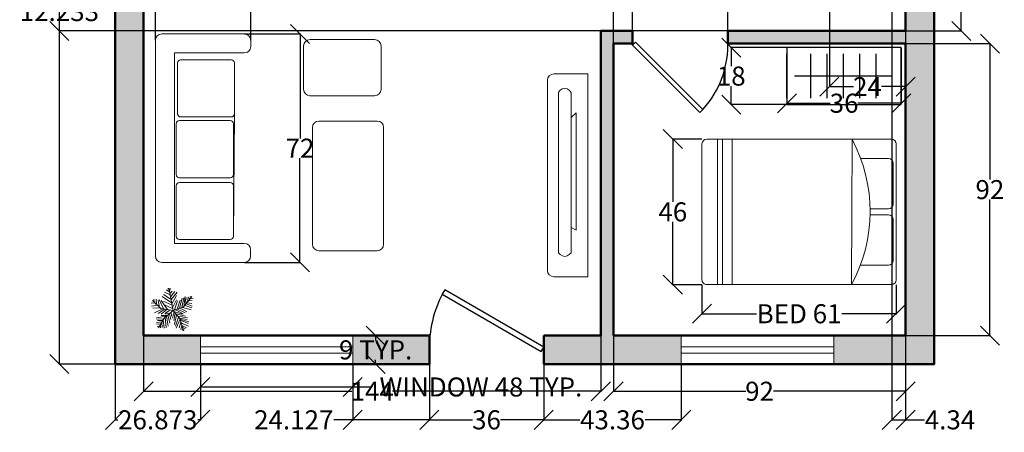
# Model space of a CAD drawing. Units: inches. Extents: x -29 to 284, y -310 to 51.
# Tile 1 of 4: x -29 to 281, y -310 to -180. Entities that reach past the tile are written whole.
import ezdxf

# ---------------------------------------------------------------- set-up
doc = ezdxf.new("R2010")
doc.units = ezdxf.units.IN
doc.header["$MEASUREMENT"] = 0
for name, color, linetype, lineweight in [('A-ANNO-DIMS', 2, 'Continuous', 18), ('A-DOOR', 3, 'Continuous', 25), ('A-EQPM', 8, 'Continuous', 18), ('A-FLOR-CASE', 9, 'Continuous', 25), ('A-FURN', 8, 'Continuous', 18), ('A-GLAZ', 4, 'Continuous', 18), ('A-WALL', 7, 'Continuous', 50)]:
    doc.layers.add(name, color=color, linetype=linetype, lineweight=lineweight)
doc.layers.add('A-WALL-PATT', color=18, linetype='Continuous', lineweight=13, true_color=0x000000)
doc.styles.get("Standard").update_dxf_attribs({"font": 'arial.ttf'})
doc.dimstyles.get("Standard").update_dxf_attribs({"dimtxt": 6, "dimasz": 6, "dimexe": 0.18, "dimexo": 0.0625, "dimgap": 0.09, "dimtad": 0, "dimtih": 1, "dimtoh": 1, "dimdec": 0, "dimzin": 0, "dimdsep": 46, "dimlunit": 4, "dimtxsty": 'Standard', "dimblk": 'OBLIQUE', "dimcen": 0.09, "dimadec": 0, "dimazin": 0, "dimtfac": 1, "dimtdec": 0, "dimtofl": 0, "dimtmove": 0, "dimatfit": 3, "dimldrblk": 'OBLIQUE', "dimfxl": 1, "dimtolj": 1, "dimtzin": 0, "dimarcsym": 0})

# ---------------------------------------------------------------- blocks, each defined once
blk = doc.blocks.new('Bed - Queen')
for p, q in [((2, 0), (58, 0)), ((0, -78), (0, -2)), ((8, -14.4), (8, -3.2)), ((10, -1.2), (26.8, -1.2)), ((28.8, -3.2), (28.8, -10.75)), ((31.2, -10.81), (31.2, -3.2)), ((33.2, -1.2), (50, -1.2)), ((52, -3.2), (52, -14.74)), ((60, -2), (60, -78)), ((0, -18.19), (60, -18.37)), ((0, -67.53), (60, -67.53)), ((0, -71.53), (60, -71.53)), ((0, -73.53), (60, -73.53)), ((58, -80), (2, -80))]:
    blk.add_line(p, q)
for centre, radius, start, end in [((2, -2), 2, 90, 180), ((58, -2), 2, 0, 90), ((10, -3.2), 2, 90, 180), ((26.8, -3.2), 2, 0, 90), ((33.2, -3.2), 2, 90, 180), ((50, -3.2), 2, 0, 90), ((29.83, -74.22), 63.48, 61.626, 118.0335), ((2, -78), 2, 180, 270), ((58, -78), 2, 270, 0)]:
    blk.add_arc(centre, radius, start, end)
blk = doc.blocks.new('*U16')
for p, q in [((0, 0), (0, 6)), ((40, 0), (40, 6))]:
    blk.add_line(p, q)
blk.add_lwpolyline([(0, 0), (28.28, -28.28), (29.52, -27.05), (1.24, 1.24)], close=True)
blk.add_arc((0, 0), 40, 315, 0)
blk = doc.blocks.new('*U11')
for p, q in [((0, 0), (0, -6)), ((-40, 0), (-40, -6))]:
    blk.add_line(p, q)
blk.add_lwpolyline([(0, 0), (-34.64, 20), (-35.52, 18.48), (-0.88, -1.52)], close=True)
blk.add_arc((0, 0), 40, 150, 180)
blk = doc.blocks.new('*U13')
for p, q in [((-8.737, 47.138), (-17.069, 52.711)), ((-10.186, 53.64), (-13.084, 55.962)), ((0, 0), (-10.5, 57)), ((-9.099, 51.782), (-6.563, 55.962)), ((-31.5, 4.5), (-52.5, 25.5)), ((-48.585, 21.131), (-49.309, 29.026)), ((-43.513, 28.561), (-42.427, 15.558)), ((-38.442, 26.239), (-34.819, 7.663)), ((-35.544, 28.097), (-24.314, 3.947)), ((-14.533, 2.09), (-30.834, 25.31)), ((-3.665, 19.273), (-27.574, 35.527)), ((-5.114, 28.097), (-24.676, 40.636)), ((-7.288, 39.707), (-21.778, 46.673)), ((-7.65, 43.423), (-2.578, 49.46)), ((-5.839, 35.992), (4.667, 48.067)), ((-5.114, 27.632), (10.463, 46.673)), ((-2.941, 16.486), (8.652, 37.85)), ((-1.129, 6.734), (9.014, 26.704)), ((10.101, 3.483), (17.708, 26.239)), ((16.259, 5.805), (23.142, 31.348)), ((22.055, 7.198), (27.489, 32.277)), ((27, 9), (48, 36)), ((27.127, 9.056), (31.112, 35.992)), ((31.836, 30.883), (32.561, 16.486)), ((35.096, 32.741), (37.27, 22.524)), ((38.719, 34.134), (41.979, 28.561)), ((40.53, 25.775), (48.862, 24.846)), ((43.791, 29.954), (51.036, 30.883)), ((44.153, 36.456), (45.239, 32.741)), ((-47.498, 19.737), (-55.83, 18.344)), ((-40.615, 13.7), (-55.105, 10.913)), ((-33.37, 6.269), (-52.207, 5.34)), ((-28.299, 3.483), (-47.86, -5.805)), ((-21.416, 3.018), (-38.079, -8.128)), ((0, 0), (-31.5, 4.5)), ((-15.982, 2.09), (-30.11, -9.521)), ((-24.314, 23.917), (-2.941, 13.7)), ((0, 0), (-22.5, -19.5)), ((-6.563, 1.161), (-21.416, -8.128)), ((-20.691, 13.7), (-1.129, 4.876)), ((0, 0), (27, 9)), ((0, 0), (18, -22.5)), ((3.942, 1.625), (11.187, 24.381)), ((6.478, 1.625), (26.04, -8.592)), ((11.187, 3.483), (30.749, -5.805)), ((18.07, 5.805), (35.096, -3.483)), ((24.229, 7.663), (46.688, 1.625)), ((29.662, 12.307), (48.137, 6.269)), ((33.285, 16.486), (48.862, 10.913)), ((36.183, 19.737), (48.137, 17.88)), ((-17.431, -15.094), (-42.789, -18.809)), ((-24.314, -21.596), (-42.427, -22.06)), ((-22.5, -19.5), (-37.5, -45)), ((-15.257, -12.772), (-30.11, -12.772)), ((-25.038, -23.918), (-22.865, -45.281)), ((-20.691, -18.345), (-17.793, -44.352)), ((-6.563, -5.805), (-19.967, -9.985)), ((-17.069, -15.094), (-12.721, -40.172)), ((-13.446, -11.378), (-8.737, -32.741)), ((-9.461, -8.592), (-6.201, -23.453)), ((-4.752, -3.483), (-3.665, -14.629)), ((2.493, -3.019), (-1.491, -20.202)), ((1.769, -2.555), (24.229, -9.521)), ((5.029, -6.27), (2.131, -25.775)), ((9.014, -11.378), (3.58, -35.992)), ((14.085, -16.951), (6.478, -40.172)), ((7.565, -9.056), (32.198, -14.629)), ((18.07, -22.524), (8.289, -45.745)), ((12.274, -15.094), (36.907, -18.809)), ((16.259, -19.738), (36.183, -22.989)), ((18, -22.5), (27, -52.5)), ((18.433, -22.524), (40.53, -29.026)), ((-28.299, -29.026), (-42.789, -31.348)), ((-30.834, -34.135), (-42.427, -35.528)), ((-34.457, -39.708), (-40.978, -42.494)), ((-26.849, -26.24), (-40.253, -25.775)), ((-32.646, -36.921), (-31.921, -44.352)), ((-29.023, -30.884), (-27.936, -43.887)), ((20.244, -30.419), (15.897, -44.816)), ((19.157, -25.311), (38.719, -33.206)), ((22.78, -37.85), (19.519, -48.532)), ((21.331, -32.741), (39.081, -40.636)), ((22.78, -38.314), (34.372, -44.816)), ((24.591, -45.745), (23.142, -50.854)), ((24.591, -43.423), (30.749, -47.603)), ((26.764, -49.925), (28.213, -50.854))]:
    blk.add_line(p, q)
blk = doc.blocks.new('WIN-48IN')
for p, q in [((0, 5.5), (48, 5.5)), ((0, 3.5), (48, 3.5))]:
    blk.add_line(p, q)
for points in [[(0, 0), (0, 9)], [(48, 9), (48, 0)]]:
    blk.add_lwpolyline(points)
blk = doc.blocks.new('_Oblique')
at = {"color": 0, "linetype": 'ByBlock', "lineweight": -2}
blk.add_line((-0.5, -0.5), (0.5, 0.5), dxfattribs=at)
blk = doc.blocks.new('*D21')
at = {"layer": 'A-ANNO-DIMS', "color": 0, "lineweight": -2, "transparency": 16777216}
for p, q in [((27.85, -288.63), (27.85, -295.94)), ((75.85, -288.63), (75.85, -295.94)), ((27.85, -295.76), (75.85, -295.76)), ((75.85, -295.76), (81.85, -295.76))]:
    blk.add_line(p, q, dxfattribs=at)
at = {"layer": 'Defpoints', "color": 0, "transparency": 16777216}
for p in [(27.85, -288.56), (75.85, -288.56), (75.85, -295.76)]:
    blk.add_point(p, dxfattribs=at)
at = {"layer": 'A-ANNO-DIMS', "color": 0, "lineweight": -2, "transparency": 16777216, "xscale": 6, "yscale": 6, "zscale": 6, "rotation": 180}
blk.add_blockref('_Oblique', (27.85, -295.76), dxfattribs=at)
at = {"layer": 'A-ANNO-DIMS', "color": 0, "lineweight": -2, "transparency": 16777216, "xscale": 6, "yscale": 6, "zscale": 6}
blk.add_blockref('_Oblique', (75.85, -295.76), dxfattribs=at)
at = {"layer": 'A-ANNO-DIMS', "color": 0, "transparency": 16777216, "insert": (116.22, -295.76), "char_height": 6, "attachment_point": 5}
blk.add_mtext('\\A1;WINDOW 48 TYP.', dxfattribs=at)
blk = doc.blocks.new('*D22')
at = {"layer": 'A-ANNO-DIMS', "color": 0, "lineweight": -2, "transparency": 16777216}
for p, q in [((75.92, -279.56), (83.23, -279.56)), ((83.05, -279.56), (83.05, -280.91)), ((83.05, -288.56), (83.05, -287.22)), ((75.92, -288.56), (83.23, -288.56))]:
    blk.add_line(p, q, dxfattribs=at)
at = {"layer": 'Defpoints', "color": 0, "transparency": 16777216}
for p in [(75.85, -279.56), (83.05, -279.56), (75.85, -288.56)]:
    blk.add_point(p, dxfattribs=at)
at = {"layer": 'A-ANNO-DIMS', "color": 0, "lineweight": -2, "transparency": 16777216, "xscale": 6, "yscale": 6, "zscale": 6}
for p, rotation in [((83.05, -279.56), 90), ((83.05, -288.56), 270)]:
    blk.add_blockref('_Oblique', p, dxfattribs=dict(at, rotation=rotation))
at = {"layer": 'A-ANNO-DIMS', "color": 0, "transparency": 16777216, "insert": (83.05, -284.06), "char_height": 6, "attachment_point": 5}
blk.add_mtext('\\A1;9 TYP.', dxfattribs=at)
blk = doc.blocks.new('*D27')
at = {"layer": 'A-ANNO-DIMS', "color": 0, "lineweight": -2, "transparency": 16777216}
for p, q in [((185.84, -263.58), (185.84, -272.87)), ((247.01, -263.58), (247.01, -272.87)), ((185.84, -272.69), (202.97, -272.69)), ((247.01, -272.69), (229.88, -272.69))]:
    blk.add_line(p, q, dxfattribs=at)
at = {"layer": 'Defpoints', "color": 0, "transparency": 16777216}
for p in [(185.84, -263.52), (247.01, -263.52), (247.01, -272.69)]:
    blk.add_point(p, dxfattribs=at)
at = {"layer": 'A-ANNO-DIMS', "color": 0, "lineweight": -2, "transparency": 16777216, "xscale": 6, "yscale": 6, "zscale": 6, "rotation": 180}
blk.add_blockref('_Oblique', (185.84, -272.69), dxfattribs=at)
at = {"layer": 'A-ANNO-DIMS', "color": 0, "lineweight": -2, "transparency": 16777216, "xscale": 6, "yscale": 6, "zscale": 6}
blk.add_blockref('_Oblique', (247.01, -272.69), dxfattribs=at)
at = {"layer": 'A-ANNO-DIMS', "color": 0, "transparency": 16777216, "insert": (216.43, -272.69), "char_height": 6, "attachment_point": 5}
blk.add_mtext('\\A1;BED 61', dxfattribs=at)
blk = doc.blocks.new('*D28')
at = {"layer": 'A-ANNO-DIMS', "color": 0, "lineweight": -2, "transparency": 16777216}
for p, q in [((185.78, -217.63), (176.48, -217.63)), ((176.66, -217.63), (176.66, -237.42)), ((176.66, -263.52), (176.66, -243.73)), ((185.78, -263.52), (176.48, -263.52))]:
    blk.add_line(p, q, dxfattribs=at)
at = {"layer": 'Defpoints', "color": 0, "transparency": 16777216}
for p in [(185.84, -217.63), (176.66, -263.52), (185.84, -263.52)]:
    blk.add_point(p, dxfattribs=at)
at = {"layer": 'A-ANNO-DIMS', "color": 0, "lineweight": -2, "transparency": 16777216, "xscale": 6, "yscale": 6, "zscale": 6}
for p, rotation in [((176.66, -217.63), 90), ((176.66, -263.52), 270)]:
    blk.add_blockref('_Oblique', p, dxfattribs=dict(at, rotation=rotation))
at = {"layer": 'A-ANNO-DIMS', "color": 0, "transparency": 16777216, "insert": (176.66, -240.57), "char_height": 6, "attachment_point": 5}
blk.add_mtext('\\A1;46', dxfattribs=at)
blk = doc.blocks.new('*D46')
at = {"layer": 'A-ANNO-DIMS', "color": 0, "lineweight": -2, "transparency": 16777216}
for p, q in [((0.92, 29.44), (-16.75, 29.44)), ((-16.57, 29.44), (-16.57, -126.41)), ((-16.57, -288.56), (-16.57, -132.72)), ((0.92, -288.56), (-16.75, -288.56))]:
    blk.add_line(p, q, dxfattribs=at)
at = {"layer": 'Defpoints', "color": 0, "transparency": 16777216}
for p in [(-16.57, 29.44), (0.98, 29.44), (0.98, -288.56)]:
    blk.add_point(p, dxfattribs=at)
at = {"layer": 'A-ANNO-DIMS', "color": 0, "lineweight": -2, "transparency": 16777216, "xscale": 6, "yscale": 6, "zscale": 6}
for p, rotation in [((-16.57, 29.44), 90), ((-16.57, -288.56), 270)]:
    blk.add_blockref('_Oblique', p, dxfattribs=dict(at, rotation=rotation))
at = {"layer": 'A-ANNO-DIMS', "color": 0, "transparency": 16777216, "insert": (-16.57, -129.56), "char_height": 6, "attachment_point": 5}
blk.add_mtext('\\A1;318', dxfattribs=at)
blk = doc.blocks.new('*D63')
at = {"layer": 'A-ANNO-DIMS', "color": 0, "lineweight": -2, "transparency": 16777216}
for p, q in [((225.98, -183.63), (225.98, -201.29)), ((249.98, -183.63), (249.98, -201.29)), ((225.98, -201.11), (233.55, -201.11)), ((249.98, -201.11), (242.41, -201.11))]:
    blk.add_line(p, q, dxfattribs=at)
at = {"layer": 'Defpoints', "color": 0, "transparency": 16777216}
for p in [(225.98, -183.56), (249.98, -183.56), (225.98, -201.11)]:
    blk.add_point(p, dxfattribs=at)
at = {"layer": 'A-ANNO-DIMS', "color": 0, "lineweight": -2, "transparency": 16777216, "xscale": 6, "yscale": 6, "zscale": 6, "rotation": 180.0000000000002}
blk.add_blockref('_Oblique', (225.98, -201.11), dxfattribs=at)
at = {"layer": 'A-ANNO-DIMS', "color": 0, "lineweight": -2, "transparency": 16777216, "xscale": 6, "yscale": 6, "zscale": 6}
blk.add_blockref('_Oblique', (249.98, -201.11), dxfattribs=at)
at = {"layer": 'A-ANNO-DIMS', "color": 0, "transparency": 16777216, "insert": (237.98, -201.11), "char_height": 6, "attachment_point": 5}
blk.add_mtext('\\A1;24', dxfattribs=at)
blk = doc.blocks.new('*D65')
at = {"layer": 'A-ANNO-DIMS', "color": 0, "lineweight": -2, "transparency": 16777216}
for p, q in [((250.04, -103.56), (267.71, -103.56)), ((267.53, -103.56), (267.53, -140.41)), ((267.53, -183.56), (267.53, -146.72)), ((250.04, -183.56), (267.71, -183.56))]:
    blk.add_line(p, q, dxfattribs=at)
at = {"layer": 'Defpoints', "color": 0, "transparency": 16777216}
for p in [(249.98, -103.56), (249.98, -183.56), (267.53, -183.56)]:
    blk.add_point(p, dxfattribs=at)
at = {"layer": 'A-ANNO-DIMS', "color": 0, "lineweight": -2, "transparency": 16777216, "xscale": 6, "yscale": 6, "zscale": 6}
for p, rotation in [((267.53, -103.56), 90), ((267.53, -183.56), 270)]:
    blk.add_blockref('_Oblique', p, dxfattribs=dict(at, rotation=rotation))
at = {"layer": 'A-ANNO-DIMS', "color": 0, "transparency": 16777216, "insert": (267.53, -143.56), "char_height": 6, "attachment_point": 5}
blk.add_mtext('\\A1;80', dxfattribs=at)
blk = doc.blocks.new('*D67')
at = {"layer": 'A-ANNO-DIMS', "color": 0, "lineweight": -2, "transparency": 16777216}
for p, q in [((228.27, -171.33), (-16.75, -171.33)), ((-16.57, -171.33), (-16.57, -174.29)), ((-16.57, -183.56), (-16.57, -180.6)), ((225.92, -183.56), (-16.75, -183.56))]:
    blk.add_line(p, q, dxfattribs=at)
at = {"layer": 'Defpoints', "color": 0, "transparency": 16777216}
for p in [(228.33, -171.33), (-16.57, -183.56), (225.98, -183.56)]:
    blk.add_point(p, dxfattribs=at)
at = {"layer": 'A-ANNO-DIMS', "color": 0, "lineweight": -2, "transparency": 16777216, "xscale": 6, "yscale": 6, "zscale": 6}
for p, rotation in [((-16.57, -171.33), 90), ((-16.57, -183.56), 270)]:
    blk.add_blockref('_Oblique', p, dxfattribs=dict(at, rotation=rotation))
at = {"layer": 'A-ANNO-DIMS', "color": 0, "transparency": 16777216, "insert": (-16.57, -177.45), "char_height": 6, "attachment_point": 5}
blk.add_mtext('\\A1;12.233', dxfattribs=at)
blk = doc.blocks.new('*D69')
at = {"layer": 'A-ANNO-DIMS', "color": 0, "lineweight": -2, "transparency": 16777216}
for p, q in [((249.98, -138.72), (249.98, -306.29)), ((245.64, -149.76), (245.64, -306.29)), ((245.64, -306.11), (249.98, -306.11)), ((249.98, -306.11), (255.98, -306.11))]:
    blk.add_line(p, q, dxfattribs=at)
at = {"layer": 'Defpoints', "color": 0, "transparency": 16777216}
for p in [(249.98, -138.66), (245.64, -149.7), (249.98, -306.11)]:
    blk.add_point(p, dxfattribs=at)
at = {"layer": 'A-ANNO-DIMS', "color": 0, "lineweight": -2, "transparency": 16777216, "xscale": 6, "yscale": 6, "zscale": 6, "rotation": 180}
blk.add_blockref('_Oblique', (245.64, -306.11), dxfattribs=at)
at = {"layer": 'A-ANNO-DIMS', "color": 0, "lineweight": -2, "transparency": 16777216, "xscale": 6, "yscale": 6, "zscale": 6}
blk.add_blockref('_Oblique', (249.98, -306.11), dxfattribs=at)
at = {"layer": 'A-ANNO-DIMS', "color": 0, "transparency": 16777216, "insert": (263.97, -306.11), "char_height": 6, "attachment_point": 5}
blk.add_mtext('\\A1;4.34', dxfattribs=at)
blk = doc.blocks.new('*D70')
at = {"layer": 'A-ANNO-DIMS', "color": 0, "lineweight": -2, "transparency": 16777216}
for p, q in [((157.98, -279.63), (157.98, -297.29)), ((249.98, -279.63), (249.98, -297.29)), ((157.98, -297.11), (199.62, -297.11)), ((249.98, -297.11), (208.34, -297.11))]:
    blk.add_line(p, q, dxfattribs=at)
at = {"layer": 'Defpoints', "color": 0, "transparency": 16777216}
for p in [(157.98, -279.56), (249.98, -279.56), (157.98, -297.11)]:
    blk.add_point(p, dxfattribs=at)
at = {"layer": 'A-ANNO-DIMS', "color": 0, "lineweight": -2, "transparency": 16777216, "xscale": 6, "yscale": 6, "zscale": 6, "rotation": 180}
blk.add_blockref('_Oblique', (157.98, -297.11), dxfattribs=at)
at = {"layer": 'A-ANNO-DIMS', "color": 0, "lineweight": -2, "transparency": 16777216, "xscale": 6, "yscale": 6, "zscale": 6}
blk.add_blockref('_Oblique', (249.98, -297.11), dxfattribs=at)
at = {"layer": 'A-ANNO-DIMS', "color": 0, "transparency": 16777216, "insert": (203.98, -297.11), "char_height": 6, "attachment_point": 5}
blk.add_mtext('\\A1;92', dxfattribs=at)
blk = doc.blocks.new('*D71')
at = {"layer": 'A-ANNO-DIMS', "color": 0, "lineweight": -2, "transparency": 16777216}
for p, q in [((9.98, -279.63), (9.98, -297.29)), ((153.98, -279.63), (153.98, -297.29)), ((9.98, -297.11), (75.56, -297.11)), ((153.98, -297.11), (88.4, -297.11))]:
    blk.add_line(p, q, dxfattribs=at)
at = {"layer": 'Defpoints', "color": 0, "transparency": 16777216}
for p in [(9.98, -279.56), (153.98, -279.56), (9.98, -297.11)]:
    blk.add_point(p, dxfattribs=at)
at = {"layer": 'A-ANNO-DIMS', "color": 0, "lineweight": -2, "transparency": 16777216, "xscale": 6, "yscale": 6, "zscale": 6, "rotation": 180}
blk.add_blockref('_Oblique', (9.98, -297.11), dxfattribs=at)
at = {"layer": 'A-ANNO-DIMS', "color": 0, "lineweight": -2, "transparency": 16777216, "xscale": 6, "yscale": 6, "zscale": 6}
blk.add_blockref('_Oblique', (153.98, -297.11), dxfattribs=at)
at = {"layer": 'A-ANNO-DIMS', "color": 0, "transparency": 16777216, "insert": (81.98, -297.11), "char_height": 6, "attachment_point": 5}
blk.add_mtext('\\A1;144', dxfattribs=at)
blk = doc.blocks.new('*D72')
at = {"layer": 'A-ANNO-DIMS', "color": 0, "lineweight": -2, "transparency": 16777216}
for p, q in [((250.04, -187.56), (276.71, -187.56)), ((276.53, -187.56), (276.53, -230.41)), ((276.53, -279.56), (276.53, -236.72)), ((250.04, -279.56), (276.71, -279.56))]:
    blk.add_line(p, q, dxfattribs=at)
at = {"layer": 'Defpoints', "color": 0, "transparency": 16777216}
for p in [(249.98, -187.56), (276.53, -187.56), (249.98, -279.56)]:
    blk.add_point(p, dxfattribs=at)
at = {"layer": 'A-ANNO-DIMS', "color": 0, "lineweight": -2, "transparency": 16777216, "xscale": 6, "yscale": 6, "zscale": 6}
for p, rotation in [((276.53, -187.56), 90), ((276.53, -279.56), 270)]:
    blk.add_blockref('_Oblique', p, dxfattribs=dict(at, rotation=rotation))
at = {"layer": 'A-ANNO-DIMS', "color": 0, "transparency": 16777216, "insert": (276.53, -233.56), "char_height": 6, "attachment_point": 5}
blk.add_mtext('\\A1;92', dxfattribs=at)
blk = doc.blocks.new('*D73')
at = {"layer": 'A-ANNO-DIMS', "color": 0, "lineweight": -2, "transparency": 16777216}
for p, q in [((157.98, -187.5), (157.98, -169.83)), ((157.98, -170.01), (158.91, -170.01)), ((163.98, -170.01), (163.05, -170.01)), ((163.98, -187.5), (163.98, -169.83))]:
    blk.add_line(p, q, dxfattribs=at)
at = {"layer": 'Defpoints', "color": 0, "transparency": 16777216}
for p in [(163.98, -170.01), (157.98, -187.56), (163.98, -187.56)]:
    blk.add_point(p, dxfattribs=at)
at = {"layer": 'A-ANNO-DIMS', "color": 0, "lineweight": -2, "transparency": 16777216, "xscale": 6, "yscale": 6, "zscale": 6, "rotation": 180}
blk.add_blockref('_Oblique', (157.98, -170.01), dxfattribs=at)
at = {"layer": 'A-ANNO-DIMS', "color": 0, "lineweight": -2, "transparency": 16777216, "xscale": 6, "yscale": 6, "zscale": 6}
blk.add_blockref('_Oblique', (163.98, -170.01), dxfattribs=at)
at = {"layer": 'A-ANNO-DIMS', "color": 0, "transparency": 16777216, "insert": (160.98, -170.01), "char_height": 6, "attachment_point": 5}
blk.add_mtext('\\A1;6', dxfattribs=at)
blk = doc.blocks.new('*D74')
at = {"layer": 'A-ANNO-DIMS', "color": 0, "lineweight": -2, "transparency": 16777216}
for p, q in [((163.98, -187.5), (163.98, -169.83)), ((163.98, -170.01), (174.61, -170.01)), ((193.98, -170.01), (183.36, -170.01)), ((193.98, -187.5), (193.98, -169.83))]:
    blk.add_line(p, q, dxfattribs=at)
at = {"layer": 'Defpoints', "color": 0, "transparency": 16777216}
for p in [(193.98, -170.01), (163.98, -187.56), (193.98, -187.56)]:
    blk.add_point(p, dxfattribs=at)
at = {"layer": 'A-ANNO-DIMS', "color": 0, "lineweight": -2, "transparency": 16777216, "xscale": 6, "yscale": 6, "zscale": 6, "rotation": 180}
blk.add_blockref('_Oblique', (163.98, -170.01), dxfattribs=at)
at = {"layer": 'A-ANNO-DIMS', "color": 0, "lineweight": -2, "transparency": 16777216, "xscale": 6, "yscale": 6, "zscale": 6}
blk.add_blockref('_Oblique', (193.98, -170.01), dxfattribs=at)
at = {"layer": 'A-ANNO-DIMS', "color": 0, "transparency": 16777216, "insert": (178.98, -170.01), "char_height": 6, "attachment_point": 5}
blk.add_mtext('\\A1;30', dxfattribs=at)
blk = doc.blocks.new('*D75')
at = {"layer": 'A-ANNO-DIMS', "color": 0, "lineweight": -2, "transparency": 16777216}
for p, q in [((0.98, -288.63), (0.98, -306.29)), ((27.85, -288.63), (27.85, -306.29)), ((0.98, -306.11), (1.82, -306.11)), ((27.85, -306.11), (27.01, -306.11))]:
    blk.add_line(p, q, dxfattribs=at)
at = {"layer": 'Defpoints', "color": 0, "transparency": 16777216}
for p in [(0.98, -288.56), (27.85, -288.56), (0.98, -306.11)]:
    blk.add_point(p, dxfattribs=at)
at = {"layer": 'A-ANNO-DIMS', "color": 0, "lineweight": -2, "transparency": 16777216, "xscale": 6, "yscale": 6, "zscale": 6, "rotation": 180.0000000000001}
blk.add_blockref('_Oblique', (0.98, -306.11), dxfattribs=at)
at = {"layer": 'A-ANNO-DIMS', "color": 0, "lineweight": -2, "transparency": 16777216, "xscale": 6, "yscale": 6, "zscale": 6}
blk.add_blockref('_Oblique', (27.85, -306.11), dxfattribs=at)
at = {"layer": 'A-ANNO-DIMS', "color": 0, "transparency": 16777216, "insert": (14.42, -306.11), "char_height": 6, "attachment_point": 5}
blk.add_mtext('\\A1;26.873', dxfattribs=at)
blk = doc.blocks.new('*D76')
at = {"layer": 'A-ANNO-DIMS', "color": 0, "lineweight": -2, "transparency": 16777216}
for p, q in [((75.85, -288.63), (75.85, -306.29)), ((99.98, -288.63), (99.98, -306.29)), ((75.85, -306.11), (69.85, -306.11)), ((99.98, -306.11), (75.85, -306.11))]:
    blk.add_line(p, q, dxfattribs=at)
at = {"layer": 'Defpoints', "color": 0, "transparency": 16777216}
for p in [(75.85, -288.56), (99.98, -288.56), (75.85, -306.11)]:
    blk.add_point(p, dxfattribs=at)
at = {"layer": 'A-ANNO-DIMS', "color": 0, "lineweight": -2, "transparency": 16777216, "xscale": 6, "yscale": 6, "zscale": 6, "rotation": 180.0000000000001}
blk.add_blockref('_Oblique', (75.85, -306.11), dxfattribs=at)
at = {"layer": 'A-ANNO-DIMS', "color": 0, "lineweight": -2, "transparency": 16777216, "xscale": 6, "yscale": 6, "zscale": 6}
blk.add_blockref('_Oblique', (99.98, -306.11), dxfattribs=at)
at = {"layer": 'A-ANNO-DIMS', "color": 0, "transparency": 16777216, "insert": (57.26, -306.11), "char_height": 6, "attachment_point": 5}
blk.add_mtext('\\A1;24.127', dxfattribs=at)
blk = doc.blocks.new('*D77')
at = {"layer": 'A-ANNO-DIMS', "color": 0, "lineweight": -2, "transparency": 16777216}
for p, q in [((99.98, -288.63), (99.98, -306.29)), ((135.98, -288.63), (135.98, -306.29)), ((99.98, -306.11), (113.6, -306.11)), ((135.98, -306.11), (122.36, -306.11))]:
    blk.add_line(p, q, dxfattribs=at)
at = {"layer": 'Defpoints', "color": 0, "transparency": 16777216}
for p in [(99.98, -288.56), (135.98, -288.56), (99.98, -306.11)]:
    blk.add_point(p, dxfattribs=at)
at = {"layer": 'A-ANNO-DIMS', "color": 0, "lineweight": -2, "transparency": 16777216, "xscale": 6, "yscale": 6, "zscale": 6, "rotation": 180}
blk.add_blockref('_Oblique', (99.98, -306.11), dxfattribs=at)
at = {"layer": 'A-ANNO-DIMS', "color": 0, "lineweight": -2, "transparency": 16777216, "xscale": 6, "yscale": 6, "zscale": 6}
blk.add_blockref('_Oblique', (135.98, -306.11), dxfattribs=at)
at = {"layer": 'A-ANNO-DIMS', "color": 0, "transparency": 16777216, "insert": (117.98, -306.11), "char_height": 6, "attachment_point": 5}
blk.add_mtext('\\A1;36', dxfattribs=at)
blk = doc.blocks.new('*D78')
at = {"layer": 'A-ANNO-DIMS', "color": 0, "lineweight": -2, "transparency": 16777216}
for p, q in [((135.98, -288.63), (135.98, -306.29)), ((179.34, -288.63), (179.34, -306.29)), ((135.98, -306.11), (147.33, -306.11)), ((179.34, -306.11), (167.99, -306.11))]:
    blk.add_line(p, q, dxfattribs=at)
at = {"layer": 'Defpoints', "color": 0, "transparency": 16777216}
for p in [(135.98, -288.56), (179.34, -288.56), (135.98, -306.11)]:
    blk.add_point(p, dxfattribs=at)
at = {"layer": 'A-ANNO-DIMS', "color": 0, "lineweight": -2, "transparency": 16777216, "xscale": 6, "yscale": 6, "zscale": 6}
for p, rotation in [((135.98, -306.11), 179.9999999999999), ((179.34, -306.11), 359.9999999999999)]:
    blk.add_blockref('_Oblique', p, dxfattribs=dict(at, rotation=rotation))
at = {"layer": 'A-ANNO-DIMS', "color": 0, "transparency": 16777216, "insert": (157.66, -306.11), "char_height": 6, "attachment_point": 5}
blk.add_mtext('\\A1;43.36', dxfattribs=at)
blk = doc.blocks.new('*D79')
at = {"layer": 'A-ANNO-DIMS', "color": 0, "lineweight": -2, "transparency": 16777216}
for p, q in [((41.75, -184.49), (59.42, -184.5)), ((59.24, -184.5), (59.23, -217.4)), ((59.21, -256.5), (59.22, -223.6)), ((41.72, -256.49), (59.39, -256.5))]:
    blk.add_line(p, q, dxfattribs=at)
at = {"layer": 'Defpoints', "color": 0, "transparency": 16777216}
for p in [(41.69, -184.49), (41.66, -256.49), (59.21, -256.5)]:
    blk.add_point(p, dxfattribs=at)
at = {"layer": 'A-ANNO-DIMS', "color": 0, "lineweight": -2, "transparency": 16777216, "xscale": 6, "yscale": 6, "zscale": 6}
for p, rotation in [((59.24, -184.5), 89.97493290739972), ((59.21, -256.5), 269.9749329073998)]:
    blk.add_blockref('_Oblique', p, dxfattribs=dict(at, rotation=rotation))
at = {"layer": 'A-ANNO-DIMS', "color": 0, "transparency": 16777216, "insert": (59.23, -220.5), "char_height": 6, "attachment_point": 5}
blk.add_mtext('\\A1;72', dxfattribs=at)
blk = doc.blocks.new('*D80')
at = {"layer": 'A-ANNO-DIMS', "color": 0, "lineweight": -2, "transparency": 16777216}
for p, q in [((13.69, -186.43), (13.69, -168.76)), ((13.69, -168.94), (24.32, -168.94)), ((43.69, -168.94), (33.07, -168.94)), ((43.69, -186.43), (43.69, -168.76))]:
    blk.add_line(p, q, dxfattribs=at)
at = {"layer": 'Defpoints', "color": 0, "transparency": 16777216}
for p in [(43.69, -168.94), (13.69, -186.49), (43.69, -186.49)]:
    blk.add_point(p, dxfattribs=at)
at = {"layer": 'A-ANNO-DIMS', "color": 0, "lineweight": -2, "transparency": 16777216, "xscale": 6, "yscale": 6, "zscale": 6, "rotation": 180}
blk.add_blockref('_Oblique', (13.69, -168.94), dxfattribs=at)
at = {"layer": 'A-ANNO-DIMS', "color": 0, "lineweight": -2, "transparency": 16777216, "xscale": 6, "yscale": 6, "zscale": 6}
blk.add_blockref('_Oblique', (43.69, -168.94), dxfattribs=at)
at = {"layer": 'A-ANNO-DIMS', "color": 0, "transparency": 16777216, "insert": (28.69, -168.94), "char_height": 6, "attachment_point": 5}
blk.add_mtext('\\A1;30', dxfattribs=at)
blk = doc.blocks.new('*D81')
at = {"layer": 'A-ANNO-DIMS', "color": 0, "lineweight": -2, "transparency": 16777216}
for p, q in [((212.6, -188.84), (212.6, -206.51)), ((248.6, -188.84), (248.6, -206.51)), ((212.6, -206.33), (226.21, -206.33)), ((248.6, -206.33), (234.98, -206.33))]:
    blk.add_line(p, q, dxfattribs=at)
at = {"layer": 'Defpoints', "color": 0, "transparency": 16777216}
for p in [(212.6, -188.78), (248.6, -188.78), (212.6, -206.33)]:
    blk.add_point(p, dxfattribs=at)
at = {"layer": 'A-ANNO-DIMS', "color": 0, "lineweight": -2, "transparency": 16777216, "xscale": 6, "yscale": 6, "zscale": 6, "rotation": 180}
blk.add_blockref('_Oblique', (212.6, -206.33), dxfattribs=at)
at = {"layer": 'A-ANNO-DIMS', "color": 0, "lineweight": -2, "transparency": 16777216, "xscale": 6, "yscale": 6, "zscale": 6}
blk.add_blockref('_Oblique', (248.6, -206.33), dxfattribs=at)
at = {"layer": 'A-ANNO-DIMS', "color": 0, "transparency": 16777216, "insert": (230.6, -206.33), "char_height": 6, "attachment_point": 5}
blk.add_mtext('\\A1;36', dxfattribs=at)
blk = doc.blocks.new('*D82')
at = {"layer": 'A-ANNO-DIMS', "color": 0, "lineweight": -2, "transparency": 16777216}
for p, q in [((212.54, -188.78), (194.87, -188.78)), ((195.05, -188.78), (195.05, -194.63)), ((195.05, -206.78), (195.05, -200.93)), ((212.54, -206.78), (194.87, -206.78))]:
    blk.add_line(p, q, dxfattribs=at)
at = {"layer": 'Defpoints', "color": 0, "transparency": 16777216}
for p in [(195.05, -188.78), (212.6, -188.78), (212.6, -206.78)]:
    blk.add_point(p, dxfattribs=at)
at = {"layer": 'A-ANNO-DIMS', "color": 0, "lineweight": -2, "transparency": 16777216, "xscale": 6, "yscale": 6, "zscale": 6}
for p, rotation in [((195.05, -188.78), 90), ((195.05, -206.78), 270)]:
    blk.add_blockref('_Oblique', p, dxfattribs=dict(at, rotation=rotation))
at = {"layer": 'A-ANNO-DIMS', "color": 0, "transparency": 16777216, "insert": (195.05, -197.78), "char_height": 6, "attachment_point": 5}
blk.add_mtext('\\A1;18', dxfattribs=at)

msp = doc.modelspace()

# ---------------------------------------------------------------- hatches: boundary and pattern name
at = {"layer": 'A-WALL-PATT'}
h = msp.add_hatch(color=256, dxfattribs=at)
h.dxf.hatch_style = 1
h.paths.add_polyline_path([(9.9809, -167.5635), (73.9809, -167.5635), (73.9809, -163.5635), (73.9809, -148.5635), (69.9809, -148.5635), (69.9809, -163.5635), (9.9809, -163.5635), (9.9809, -144.6496), (0.9809, -144.6496), (0.9809, -288.5635), (27.8543, -288.5635), (27.8543, -279.5635), (9.9809, -279.5635)])
h = msp.add_hatch(color=256, dxfattribs=at)
h.dxf.hatch_style = 1
h.paths.add_polyline_path([(258.9809, -162.6614), (249.9809, -162.6614), (249.9809, -183.5635), (193.9809, -183.5635), (193.9809, -187.5635), (249.9809, -187.5635), (249.9809, -279.5635), (227.3376, -279.5635), (227.3376, -288.5635), (258.9809, -288.5635)])
h = msp.add_hatch(color=256, dxfattribs=at)
h.dxf.hatch_style = 1
h.paths.add_polyline_path([(157.9809, -279.5635), (157.9809, -187.5635), (163.9809, -187.5635), (163.9809, -183.5635), (153.9809, -183.5635), (153.9809, -279.5635), (135.9809, -279.5635), (135.9809, -288.5635), (179.3376, -288.5635), (179.3376, -279.5635)])
h = msp.add_hatch(color=256, dxfattribs=at)
h.dxf.hatch_style = 1
h.paths.add_polyline_path([(99.9809, -283.1635), (99.9809, -279.5635), (75.8543, -279.5635), (75.8543, -288.5635), (99.9809, -288.5635)])

# ---------------------------------------------------------------- linework, layer by layer
at = {"layer": 'A-EQPM'}
for p, q in [((140.6343, -202.8294), (141.1934, -202.2703)), ((144.0218, -202.2703), (144.581, -202.8294)), ((146.2211, -209.3595), (144.6049, -210.7997)), ((146.2211, -246.3453), (144.6049, -245.4963)), ((140.6463, -253.4737), (141.2062, -254.0336)), ((144.6049, -253.4737), (144.0217, -254.0463))]:
    msp.add_line(p, q, dxfattribs=at)
for points in [[(140.6343, -202.8294), (140.6104, -202.8294), (140.6104, -253.4737), (140.6463, -253.4737)], [(144.569, -253.4737), (144.6049, -253.4737), (144.6049, -202.8294), (144.581, -202.8294)], [(144.6049, -246.3453), (144.6049, -209.3595)], [(146.2211, -209.3595), (146.2211, -246.3453)]]:
    msp.add_lwpolyline(points, dxfattribs=at)
for centre, radius, start, end in [((142.6076, -203.6845), 2, 45, 135), ((142.6204, -252.6194), 2, 225, 314.481139), ((142.6076, -253.4737), 1.9614, 358.962278, 0)]:
    msp.add_arc(centre, radius, start, end, dxfattribs=at)
at = {"layer": 'A-FLOR-CASE'}
for p, q in [((225.9809, -103.5635), (225.9809, -183.5635)), ((248.598, -188.7804), (212.598, -188.7804)), ((212.598, -188.7804), (212.598, -206.7804)), ((248.598, -206.7804), (248.598, -188.7804)), ((212.598, -204.7804), (212.598, -190.7804)), ((220.1482, -204.7804), (220.1482, -190.7804)), ((225.2911, -204.7804), (225.2911, -190.7804)), ((230.434, -204.7804), (230.434, -190.7804)), ((235.5768, -204.7804), (235.5768, -190.7804)), ((240.7197, -204.7804), (240.7197, -190.7804)), ((245.8625, -197.7804), (215.0054, -197.7804)), ((212.598, -206.7804), (248.598, -206.7804))]:
    msp.add_line(p, q, dxfattribs=at)
at = {"layer": 'A-FURN'}
for p, q in [((15.692, -184.4922), (37.692, -184.4922)), ((37.692, -184.4922), (41.692, -184.4922)), ((13.692, -254.4921), (13.692, -186.4922)), ((43.692, -186.4922), (43.692, -188.4921)), ((37.692, -190.4921), (19.692, -190.4921)), ((19.692, -190.4921), (19.692, -250.4921)), ((41.692, -190.4921), (37.692, -190.4921)), ((38.6199, -209.6521), (38.2312, -248.3066)), ((19.692, -250.4921), (37.6605, -250.4921)), ((37.6605, -250.4921), (41.6605, -250.4921)), ((43.6605, -252.4921), (43.6605, -254.4921)), ((37.692, -256.4921), (15.692, -256.4921)), ((41.6605, -256.4921), (37.6605, -256.4921))]:
    msp.add_line(p, q, dxfattribs=at)
for points in [[(62.3439, -186.2947), (82.7463, -186.2947, -0.41421356), (84.7463, -188.2947), (84.7463, -201.9674, -0.41421356), (82.7463, -203.9674), (62.3439, -203.9674, -0.41421356), (60.3439, -201.9674), (60.3439, -188.2947, -0.41421356)], [(21.6199, -192.6521), (37.6199, -192.6521, -0.41421356), (38.6199, -193.6521), (38.6199, -209.6521, -0.41421356), (37.6199, -210.6521), (21.6199, -210.6521, -0.41421356), (20.6199, -209.6521), (20.6199, -193.6521, -0.41421356)], [(149.8806, -197.0966), (139.1755, -197.0966, 0.41421356), (137.1755, -199.0966), (137.1755, -259.0416, 0.41421356), (139.1755, -261.0416), (149.8806, -261.0416)], [(21.2574, -211.8141), (37.2574, -211.8141, -0.41421356), (38.2574, -212.8141), (38.2574, -228.8141, -0.41421356), (37.2574, -229.8141), (21.2574, -229.8141, -0.41421356), (20.2574, -228.8141), (20.2574, -212.8141, -0.41421356)], [(65.1592, -211.9512), (83.5554, -211.9512, -0.41421356), (85.5554, -213.9512), (85.5554, -250.8047, -0.41421356), (83.5554, -252.8047), (65.1592, -252.8047, -0.41421356), (63.1592, -250.8047), (63.1592, -213.9512, -0.41421356)], [(21.2312, -231.3066), (37.2312, -231.3066, -0.41421356), (38.2312, -232.3066), (38.2312, -248.3066, -0.41421356), (37.2312, -249.3066), (21.2312, -249.3066, -0.41421356), (20.2312, -248.3066), (20.2312, -232.3066, -0.41421356)]]:
    msp.add_lwpolyline(points, format="xyb", close=True, dxfattribs=at)
for centre, start, end in [((15.692, -186.4922), 90, 180), ((41.692, -186.4922), 0, 90), ((41.692, -188.4921), 270, 0), ((41.6605, -252.4921), 0, 90), ((15.692, -254.4921), 180, 270), ((41.6605, -254.4921), 270, 0)]:
    msp.add_arc(centre, 2, start, end, dxfattribs=at)
at = {"layer": 'A-WALL'}
for p, q in [((249.9809, -103.5635), (249.9809, -183.5635)), ((9.9809, -279.5635), (9.9809, -167.5635)), ((153.9809, -183.5635), (153.9809, -279.5635)), ((163.9809, -183.5635), (153.9809, -183.5635)), ((163.9809, -187.5635), (163.9809, -183.5635)), ((249.9809, -183.5635), (193.9809, -183.5635)), ((193.9809, -187.5635), (193.9809, -183.5635)), ((157.9809, -187.5635), (157.9809, -279.5635)), ((163.9809, -187.5635), (157.9809, -187.5635)), ((249.9809, -187.5635), (193.9809, -187.5635)), ((249.9809, -187.5635), (249.9809, -279.5635)), ((99.9809, -279.5635), (9.9809, -279.5635)), ((99.9809, -279.5635), (99.9809, -288.5635)), ((153.9809, -279.5635), (135.9809, -279.5635)), ((153.9809, -279.5635), (135.9809, -279.5635)), ((135.9809, -279.5635), (135.9809, -288.5635)), ((249.9809, -279.5635), (157.9809, -279.5635))]:
    msp.add_line(p, q, dxfattribs=at)
msp.add_lwpolyline([(99.9809, -288.5635), (0.9809, -288.5635), (0.9809, 29.4365), (258.9809, 29.4365), (258.9809, -288.5635), (135.9809, -288.5635)], dxfattribs=at)

# ---------------------------------------------------------------- block references
at = {"layer": 'A-DOOR'}
for name, p, xscale, yscale, zscale in [('*U16', (163.9809, -188.0635), 0.75, 0.75, 0.75), ('*U11', (135.9809, -283.1635), 0.8999999999999976, 0.8999999999999976, 0.8999999999999976)]:
    msp.add_blockref(name, p, dxfattribs=dict(at, xscale=xscale, yscale=yscale, zscale=zscale))
at = {"layer": 'A-FURN', "xscale": 0.7647023752056115, "yscale": 0.7647023752056115, "zscale": 0.7647023752056115, "rotation": 270}
msp.add_blockref('Bed - Queen', (247.0146, -217.6334), dxfattribs=at)
at = {"layer": 'A-FURN', "xscale": 0.1230009303838199, "yscale": 0.1230009303838199, "zscale": 0.1230009303838199}
msp.add_blockref('*U13', (19.2536, -271.6285), dxfattribs=at)
at = {"layer": 'A-GLAZ'}
for p in [(27.8544, -288.563), (179.3376, -288.563)]:
    msp.add_blockref('WIN-48IN', p, dxfattribs=at)

# ---------------------------------------------------------------- dimensions: what is measured, and where the dimension line sits
at = {"layer": 'A-ANNO-DIMS'}
for base, p1, p2, angle, override, picture, middle in [((-16.5691, 29.4365), (0.9809, -288.5635), (0.9809, 29.4365), 90, {"dimdec": 0, "dimlfac": 1, "dimrnd": 0, "dimzin": 0, "dimdsep": 46, "dimlunit": 2}, '*D46', (-16.5691, -129.5635)), ((267.5309, -183.5635), (249.9809, -103.5635), (249.9809, -183.5635), 270, {"dimdec": 0, "dimlfac": 1, "dimrnd": 0, "dimzin": 0, "dimdsep": 46, "dimlunit": 2}, '*D65', (267.5309, -143.5635)), ((-16.5691, -183.5635), (228.3299, -171.3301), (225.9809, -183.5635), 90, {"dimdec": 3, "dimlfac": 1, "dimrnd": 0, "dimzin": 0, "dimdsep": 46, "dimlunit": 2}, '*D67', (-16.5691, -177.4468)), ((59.2105, -256.4998), (41.692, -184.4922), (41.6605, -256.4921), 269.974933, {"dimdec": 0, "dimlfac": 1, "dimrnd": 0, "dimzin": 0, "dimdsep": 46, "dimlunit": 2}, '*D79', (59.2263, -220.4998)), ((195.048, -188.7804), (212.598, -206.7804), (212.598, -188.7804), 90, {"dimdec": 0, "dimlfac": 1, "dimrnd": 0, "dimzin": 0, "dimdsep": 46, "dimlunit": 2}, '*D82', (195.048, -197.7804)), ((225.9809, -201.1135), (249.9809, -183.5635), (225.9809, -183.5635), 180, {"dimdec": 0, "dimlfac": 1, "dimrnd": 0, "dimzin": 0, "dimdsep": 46, "dimlunit": 2}, '*D63', (237.9809, -201.1135)), ((276.5309, -187.5635), (249.9809, -279.5635), (249.9809, -187.5635), 90, {"dimdec": 0, "dimlfac": 1, "dimrnd": 0, "dimzin": 0, "dimdsep": 46, "dimlunit": 2}, '*D72', (276.5309, -233.5635)), ((212.598, -206.3304), (248.598, -188.7804), (212.598, -188.7804), 180, {"dimdec": 0, "dimlfac": 1, "dimrnd": 0, "dimzin": 0, "dimdsep": 46, "dimlunit": 2}, '*D81', (230.598, -206.3304)), ((176.662, -263.5155), (185.8384, -217.6334), (185.8384, -263.5155), 270, {"dimdec": 0, "dimlfac": 1, "dimrnd": 0, "dimzin": 0, "dimdsep": 46, "dimlunit": 2}, '*D28', (176.662, -240.5744)), ((9.9809, -297.1135), (153.9809, -279.5635), (9.9809, -279.5635), 180, {"dimdec": 0, "dimlfac": 1, "dimrnd": 0, "dimzin": 0, "dimdsep": 46, "dimlunit": 2}, '*D71', (81.9809, -297.1135)), ((157.9809, -297.1135), (249.9809, -279.5635), (157.9809, -279.5635), 180, {"dimdec": 0, "dimlfac": 1, "dimrnd": 0, "dimzin": 0, "dimdsep": 46, "dimlunit": 2}, '*D70', (203.9809, -297.1135)), ((0.9809, -306.1135), (27.8543, -288.5635), (0.9809, -288.5635), 180, {"dimdec": 3, "dimlfac": 1, "dimrnd": 0, "dimzin": 0, "dimdsep": 46, "dimlunit": 2}, '*D75', (14.4176, -306.1135)), ((75.8543, -306.1135), (99.9809, -288.5635), (75.8543, -288.5635), 180, {"dimdec": 3, "dimlfac": 1, "dimrnd": 0, "dimzin": 0, "dimdsep": 46, "dimlunit": 2}, '*D76', (57.2589, -306.1135)), ((99.9809, -306.1135), (135.9809, -288.5635), (99.9809, -288.5635), 180, {"dimdec": 0, "dimlfac": 1, "dimrnd": 0, "dimzin": 0, "dimdsep": 46, "dimlunit": 2}, '*D77', (117.9809, -306.1135)), ((135.9809, -306.1135), (179.3376, -288.5635), (135.9809, -288.5635), 180, {"dimdec": 2, "dimlfac": 1, "dimrnd": 0, "dimzin": 0, "dimdsep": 46, "dimlunit": 2}, '*D78', (157.6593, -306.1135))]:
    dim = msp.add_linear_dim(base=base, p1=p1, p2=p2, angle=angle, dimstyle='Standard', override=override, dxfattribs=at)
    dim.commit()
    dim.dimension.update_dxf_attribs({"geometry": picture, "text_midpoint": middle})
for base, p1, p2, override, picture, middle in [((249.9809, -306.1135), (245.6365, -149.6968), (249.9809, -138.6614), {"dimdec": 2, "dimlfac": 1, "dimrnd": 0, "dimzin": 0, "dimdsep": 46, "dimlunit": 2}, '*D69', (263.972, -306.1135)), ((43.692, -168.9421), (13.692, -186.4922), (43.692, -186.4922), {"dimdec": 0, "dimlfac": 1, "dimrnd": 0, "dimzin": 0, "dimdsep": 46, "dimlunit": 2}, '*D80', (28.692, -168.9421)), ((163.9809, -170.0135), (157.9809, -187.5635), (163.9809, -187.5635), {"dimdec": 0, "dimlfac": 1, "dimrnd": 0, "dimzin": 0, "dimdsep": 46, "dimlunit": 2}, '*D73', (160.9809, -170.0135)), ((193.9809, -170.0135), (163.9809, -187.5635), (193.9809, -187.5635), {"dimdec": 0, "dimlfac": 1, "dimrnd": 0, "dimzin": 0, "dimdsep": 46, "dimlunit": 2}, '*D74', (178.9809, -170.0135))]:
    dim = msp.add_linear_dim(base=base, p1=p1, p2=p2, dimstyle='Standard', override=override, dxfattribs=at)
    dim.commit()
    dim.dimension.update_dxf_attribs({"geometry": picture, "text_midpoint": middle})
for base, p1, p2, text, picture, middle in [((247.0146, -272.6919), (185.8384, -263.5155), (247.0146, -263.5155), 'BED <>', '*D27', (216.4265, -272.6919)), ((75.8543, -295.7635), (27.8543, -288.5635), (75.8543, -288.5635), 'WINDOW <> TYP.', '*D21', (116.2233, -295.7635))]:
    dim = msp.add_linear_dim(base=base, p1=p1, p2=p2, text=text, dimstyle='Standard', override={"dimdec": 0, "dimlfac": 1, "dimrnd": 0, "dimzin": 0, "dimdsep": 46, "dimlunit": 2}, dxfattribs=at)
    dim.commit()
    dim.dimension.update_dxf_attribs({"geometry": picture, "text_midpoint": middle})
dim = msp.add_linear_dim(base=(83.0543, -279.5635), p1=(75.8543, -288.5635), p2=(75.8543, -279.5635), angle=90, text='<> TYP.', dimstyle='Standard', override={"dimdec": 0, "dimlfac": 1, "dimrnd": 0, "dimzin": 0, "dimdsep": 46, "dimlunit": 2}, dxfattribs=at)
dim.commit()
dim.dimension.update_dxf_attribs({"geometry": '*D22', "text_midpoint": (83.0543, -284.0635)})

doc.saveas('drawing.dxf')
